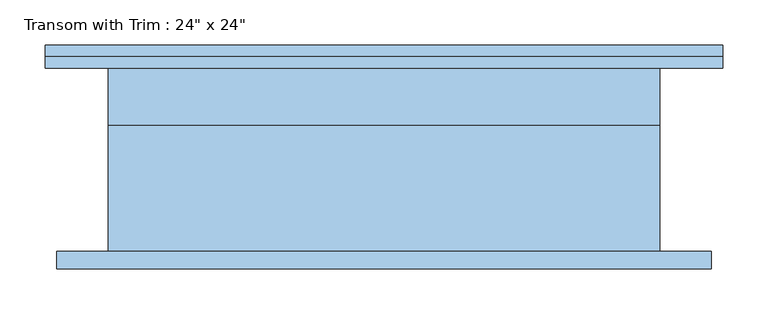
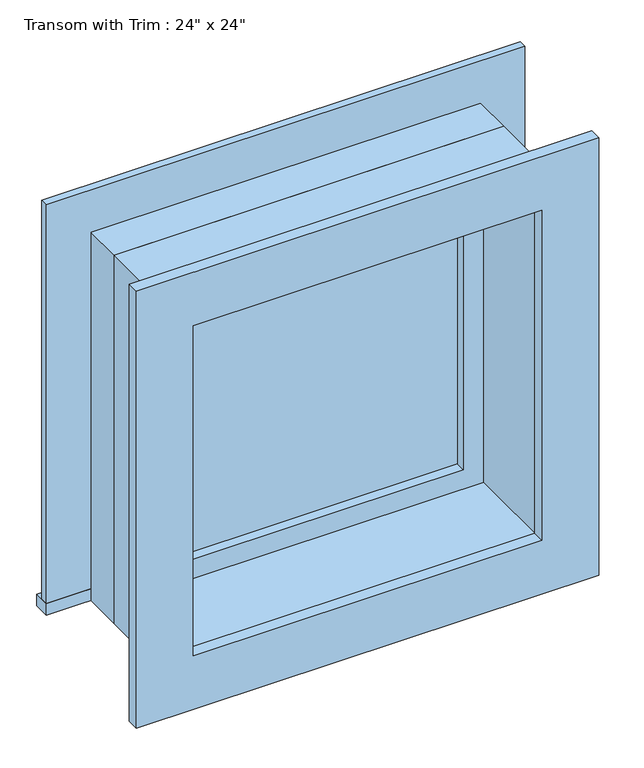
"""IFC4 building model written with IfcOpenShell, lengths in millimetres: window geometry."""

from ifc_helpers import new_model, si_unit, frame, origin, place, context, project, spatial, polyline, outline, extrude, source, transform, mapped, element, save


def window_e41d21a6(model_context):
    return source(origin(), model_context, "Body", "SweptSolid", [
        extrude(outline(polyline([(-412.75, 127.0), (336.55, 127.0), (336.55, 101.6), (-412.75, 101.6), (-412.75, 127.0)])), frame((0.0, 0.0, 2159.0), z_axis=(0.0, 0.0, 1.0), x_axis=(1.0, 0.0, 0.0)), (0.0, 0.0, 1.0), 19.05),
        extrude(outline(polyline([(2749.55, -323.85), (2749.55, 247.65), (2178.05, 247.65), (2178.05, 336.55), (2838.45, 336.55), (2838.45, -412.75), (2178.05, -412.75), (2178.05, -323.85), (2749.55, -323.85)])), frame((0.0, 101.6, 0.0), z_axis=(0.0, 1.0, 0.0), x_axis=(0.0, 0.0, 1.0)), (0.0, 0.0, 1.0), 12.7),
        extrude(outline(polyline([(2825.75, 323.85), (2825.75, -400.05), (2101.85, -400.05), (2101.85, 323.85), (2825.75, 323.85)]), holes=[polyline([(2736.85, 234.95), (2190.75, 234.95), (2190.75, -311.15), (2736.85, -311.15), (2736.85, 234.95)])]), frame((0.0, -120.65, 0.0), z_axis=(0.0, 1.0, 0.0), x_axis=(0.0, 0.0, 1.0)), (0.0, 0.0, 1.0), 19.05),
        extrude(outline(polyline([(203.2, 53.975), (-279.4, 53.975), (-279.4, 66.675), (203.2, 66.675), (203.2, 53.975)])), frame((0.0, 0.0, 2222.5), z_axis=(0.0, 0.0, 1.0), x_axis=(1.0, 0.0, 0.0)), (0.0, 0.0, 1.0), 482.6),
        extrude(outline(polyline([(2749.55, -323.85), (2178.05, -323.85), (2178.05, 247.65), (2749.55, 247.65), (2749.55, -323.85)]), holes=[polyline([(2705.1, -279.4), (2705.1, 203.2), (2222.5, 203.2), (2222.5, -279.4), (2705.1, -279.4)])]), frame((0.0, 38.1, 0.0), z_axis=(0.0, 1.0, 0.0), x_axis=(0.0, 0.0, 1.0)), (0.0, 0.0, 1.0), 44.45),
        extrude(outline(polyline([(2768.6, -342.9), (2159.0, -342.9), (2159.0, 266.7), (2768.6, 266.7), (2768.6, -342.9)]), holes=[polyline([(2736.85, -311.15), (2736.85, 234.95), (2190.75, 234.95), (2190.75, -311.15), (2736.85, -311.15)])]), frame((0.0, -101.6, 0.0), z_axis=(0.0, 1.0, 0.0), x_axis=(0.0, 0.0, 1.0)), (0.0, 0.0, 1.0), 139.7),
        extrude(outline(polyline([(2768.6, 266.7), (2768.6, -342.9), (2159.0, -342.9), (2159.0, 266.7), (2768.6, 266.7)]), holes=[polyline([(2749.55, 247.65), (2178.05, 247.65), (2178.05, -323.85), (2749.55, -323.85), (2749.55, 247.65)])]), frame((0.0, 38.1, 0.0), z_axis=(0.0, 1.0, 0.0), x_axis=(0.0, 0.0, 1.0)), (0.0, 0.0, 1.0), 63.5),
    ])


if __name__ == "__main__":
    model = new_model("IFC4")
    model_context = context("Model", 3, world=origin())
    ifc_project = project(units=[si_unit("LENGTHUNIT", "METRE", prefix="MILLI")], contexts=[model_context])
    site = spatial("IfcSite", under=ifc_project)
    building = spatial("IfcBuilding", under=site)
    placement = place(None, origin())
    window_shape = window_e41d21a6(model_context)
    element("IfcWindow", 1, ObjectType="Transom with Trim : 24\" x 24\"", at=placement, inside=building, context=model_context, shape_type="MappedRepresentation", body=[
        mapped(window_shape, transform((0.0, 0.0, 0.0), x_axis=(1.0, 0.0, 0.0), y_axis=(0.0, 1.0, 0.0), z_axis=(0.0, 0.0, 1.0))),
    ])
    save(model, "model.ifc")

# Revit data of these elements
# Type "Transom with Trim : 24\" x 24\""
#   Type Mark = "14"
#   Construction Type Id = "GSP4R"
#   Assembly Code = "B2020100"
#   Analytic Construction = "1/8 in Pilkington single glazing"
#   Visual Light Transmittance = 0.9
#   Solar Heat Gain Coefficient = 0.78
#   Heat Transfer Coefficient (U) = 0.6496 BTU/(h·ft²·°F)
#   Height = 2' - 0"
#   Default Sill Height = 7' - 1"
#   Trim Projection - Ext. = 0' - 0 1/2"
#   Trim Projection - Int. = 0' - 0 3/4"
#   Trim Width - Exterior = 0' - 3 1/2"
#   Trim Width - Interior = 0' - 3 1/2"
#   Width = 2' - 0"
#   Window Inset = 0' - 0 3/4"
#   Define Thermal Properties by = 1
#   Glass Pane Material = Glass
#   Sash Material = Sash
#   Trim Exterior Material = Trim
#   Trim Interior Material = Trim
#   Wall Closure = (empty or 0)
# Element 1 (IfcWindow, "Transom with Trim : 24\" x 24\"")
#   Materials on its faces: "Sash", "Trim", "Glass"
# Materials
#   "Glass": class "Glass", colour RGB 0 128 192, transparency 0.75, Description = "Soda Lime Glass", Cost = 0
#   "Sash": class "Wood", colour RGB 224 178 126, transparency 0
#   "Trim": class "Wood", colour RGB 224 178 126, transparency 0
